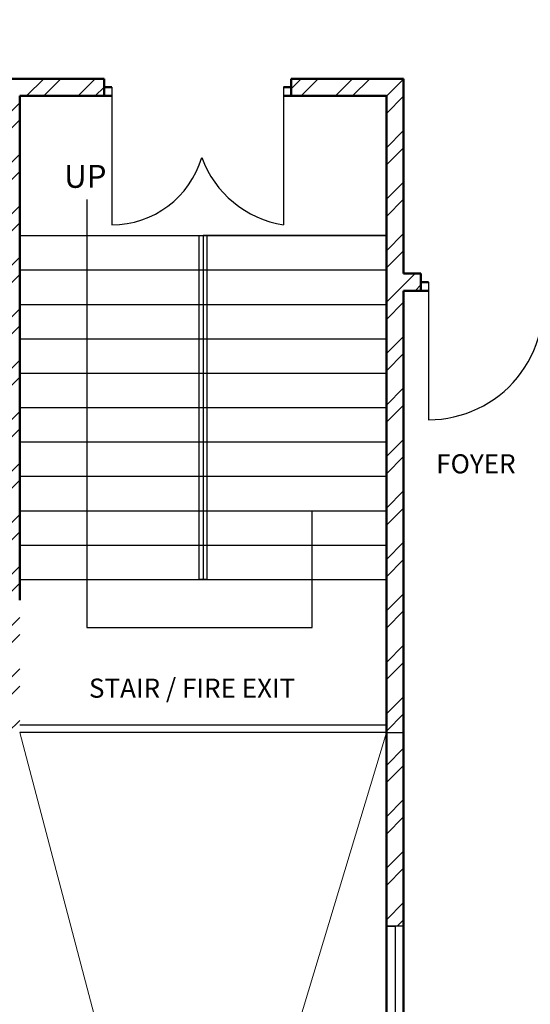
# Model space of a CAD drawing. Units: inches. Extents: x 1901 to 2863, y 888 to 2433.
# Tile 35 of 91: x 2343 to 2477, y 1474 to 1732. Entities that reach past the tile are written whole.
import ezdxf

# ---------------------------------------------------------------- set-up
doc = ezdxf.new("R2010")
doc.units = ezdxf.units.IN
for name, color, linetype, lineweight in [('A-ANNO-SYMB', 8, 'Continuous', 13), ('A-AREA-IDEN', 7, 'Continuous', 18), ('A-DOOR', 4, 'Continuous', 25), ('A-FLOR-STRS', 2, 'Continuous', 25), ('A-GLAZ', 3, 'Continuous', 25), ('A-WALL', 7, 'Continuous', 50), ('A-WALL-PATT', 8, 'Continuous', 13)]:
    doc.layers.add(name, color=color, linetype=linetype, lineweight=lineweight)
doc.styles.get("Standard").update_dxf_attribs({"font": 'arial.ttf'})

# ---------------------------------------------------------------- blocks, each defined once
blk = doc.blocks.new('WIN-60')
for p, q in [((0, 4.5), (0, 0)), ((60, 2.25), (60, 4.5)), ((60, 4.5), (60, 0)), ((0, 0), (0, 2.25)), ((0, 2.25), (60, 2.25))]:
    blk.add_line(p, q)

msp = doc.modelspace()

# ---------------------------------------------------------------- hatches: boundary and pattern name
at = {"layer": 'A-WALL-PATT'}
h = msp.add_hatch(dxfattribs=at)
h.set_pattern_fill('ANSI32', color=256)
h.paths.add_polyline_path([(2192.5, 2274.13), (2141.26, 2274.13), (2141.26, 2269.63), (2192.5, 2269.63)])
h.paths.add_polyline_path([(2259.93, 2274.13), (2216.5, 2274.13), (2216.5, 2269.63), (2255.43, 2269.63), (2255.43, 2214.63), (2250.81, 2214.63), (2250.81, 2210.13), (2259.93, 2210.13), (2259.93, 2215.13), (2271.76, 2215.13), (2271.76, 2217.38), (2271.76, 2219.63), (2259.93, 2219.63)])
h.paths.add_polyline_path([(2171.43, 2269.63), (2166.93, 2269.63), (2166.93, 2219.63), (2121.24, 2219.63), (2121.24, 2215.13), (2166.93, 2215.13), (2166.93, 2083.13), (2161.81, 2083.13), (2161.81, 2078.63), (2171.43, 2078.63), (2177, 2078.63), (2177, 2080.88), (2177, 2083.13), (2171.43, 2083.13), (2171.43, 2210.13), (2230.91, 2210.13), (2230.91, 2212.38), (2230.91, 2214.63), (2171.43, 2214.63)])
h.paths.add_polyline_path([(2117.26, 2274.13), (2089.43, 2274.13), (2089.43, 2219.63), (2081.14, 2219.63), (2081.14, 2215.13), (2089.43, 2215.13), (2098, 2215.13), (2098, 2217.38), (2098, 2219.63), (2093.93, 2219.63), (2093.93, 2269.63), (2117.26, 2269.63), (2117.26, 2271.88)])
h.paths.add_polyline_path([(2343.43, 2219.63), (2329.29, 2219.63), (2329.29, 2215.13), (2338.93, 2215.13), (2338.93, 2184.74), (2343.43, 2184.74)])
h.paths.add_polyline_path([(2338.93, 2083.13), (2329.29, 2083.13), (2208.97, 2083.13), (2208.97, 2078.63), (2338.93, 2078.63)])
h.paths.add_polyline_path([(2343.43, 2136.74), (2338.93, 2136.74), (2338.93, 1872.63), (2343.43, 1872.63)])
h.paths.add_polyline_path([(2343.43, 1863.63), (2397.68, 1863.63), (2397.68, 1821.63), (2384.14, 1821.63), (2384.14, 1812.63), (2418.33, 1812.63), (2418.33, 1817.13), (2418.33, 1821.63), (2406.68, 1821.63), (2406.68, 1863.63), (2459.5, 1863.63), (2459.5, 1821.63), (2447.14, 1821.63), (2447.14, 1812.63), (2459.5, 1812.63), (2468.5, 1812.63), (2468.5, 1872.63), (2394.43, 1872.63), (2334.43, 1872.63), (2334.43, 1812.63), (2343.43, 1812.63), (2353.25, 1812.63), (2353.25, 1821.63), (2343.43, 1821.63)])
h.paths.add_polyline_path([(2510.01, 1872.63), (2468.5, 1872.63), (2468.5, 1868.13), (2510.01, 1868.13)])
h.paths.add_polyline_path([(2514.01, 1817.13), (2468.5, 1817.13), (2468.5, 1812.63), (2482.11, 1812.63), (2482.11, 1800.61), (2486.61, 1800.61), (2486.61, 1812.63), (2514.01, 1812.63)])
h.paths.add_polyline_path([(2299.25, 1814.88), (2299.25, 1817.13), (2295.93, 1817.13), (2295.93, 1854.17), (2293.68, 1854.17), (2291.43, 1854.17), (2291.43, 1817.13), (2266.11, 1817.13), (2266.11, 1812.63), (2299.25, 1812.63)])
h.paths.add_polyline_path([(2218.11, 1817.13), (2206.46, 1817.13), (2171.43, 1817.13), (2171.43, 1949.13), (2190.1, 1949.13), (2190.1, 1953.63), (2163.47, 1953.63), (2163.47, 1949.13), (2166.93, 1949.13), (2166.93, 1817.13), (2114.3, 1817.13), (2114.3, 1812.63), (2218.11, 1812.63)])
h.paths.add_polyline_path([(2029.43, 1970.92), (2024.93, 1970.92), (2024.93, 1912.72), (2029.43, 1912.72)])
h.paths.add_polyline_path([(2132.3, 1953.63), (2113.93, 1953.63), (2113.93, 1975.89), (2111.68, 1975.89), (2109.43, 1975.89), (2109.43, 1953.63), (2029.43, 1953.63), (2029.43, 1949.13), (2132.3, 1949.13)])
h.paths.add_polyline_path([(2029.43, 1853.61), (2029.31, 1853.61), (2029.31, 1853.61), (2029.43, 1853.61), (2029.43, 1864.72), (2024.93, 1864.72), (2024.93, 1812.63), (2066.3, 1812.63), (2066.3, 1814.88), (2066.3, 1817.13), (2029.43, 1817.13)])
h.paths.add_polyline_path([(2122.93, 2010.09), (2120.68, 2010.09), (2118.43, 2010.09), (2118.43, 2006.13), (2029.43, 2006.13), (2029.43, 2001.63), (2109.43, 2001.63), (2109.43, 1998.04), (2113.93, 1998.04), (2113.93, 2001.63), (2122.93, 2001.63)])
h.paths.add_polyline_path([(2029.43, 2031.38), (2024.93, 2031.38), (2024.93, 1994.92), (2027.18, 1994.92), (2029.43, 1994.92)])
h.paths.add_polyline_path([(2029.43, 2136.74), (2024.93, 2136.74), (2024.93, 2067.38), (2027.18, 2067.38), (2029.43, 2067.38)])
h.paths.add_polyline_path([(2125.62, 2083.13), (2029.43, 2083.13), (2029.43, 2078.63), (2118.43, 2078.63), (2118.43, 2030.71), (2122.93, 2030.71), (2122.93, 2078.63), (2125.62, 2078.63)])
h.paths.add_polyline_path([(2029.43, 2215.13), (2040.47, 2215.13), (2040.47, 2217.38), (2040.47, 2219.63), (2024.93, 2219.63), (2024.93, 2184.74), (2029.43, 2184.74), (2029.43, 2187.78)])
h.paths.add_polyline_path([(2686.43, 2274.13), (2659.28, 2274.13), (2659.28, 2269.63), (2681.93, 2269.63), (2681.93, 2219.63), (2676.82, 2219.63), (2676.82, 2215.13), (2681.93, 2215.13), (2697.01, 2215.13), (2697.01, 2217.38), (2697.01, 2219.63), (2686.43, 2219.63)])
h.paths.add_polyline_path([(2609.93, 2269.63), (2635.28, 2269.63), (2635.28, 2274.13), (2571.43, 2274.13), (2571.43, 2269.63), (2605.43, 2269.63), (2605.43, 2214.63), (2549.1, 2214.63), (2549.1, 2210.13), (2605.43, 2210.13), (2605.43, 2083.13), (2601.01, 2083.13), (2601.01, 2080.88), (2601.01, 2078.63), (2609.93, 2078.63), (2616.16, 2078.63), (2616.16, 2080.88), (2616.16, 2083.13), (2609.93, 2083.13), (2609.93, 2215.13), (2651.46, 2215.13), (2651.46, 2217.38), (2651.46, 2219.63), (2609.93, 2219.63)])
h.paths.add_polyline_path([(2521.43, 2269.63), (2547.43, 2269.63), (2547.43, 2271.88), (2547.43, 2274.13), (2516.93, 2274.13), (2516.93, 2219.63), (2506.41, 2219.63), (2506.41, 2215.13), (2516.93, 2215.13), (2516.93, 2210.13), (2525.4, 2210.13), (2525.4, 2212.38), (2525.4, 2214.63), (2521.43, 2214.63)])
h.paths.add_polyline_path([(2456.01, 2219.63), (2439.43, 2219.63), (2439.43, 2187.89), (2443.93, 2187.89), (2443.93, 2215.13), (2456.01, 2215.13)])
h.paths.add_polyline_path([(2752.93, 2219.63), (2739.48, 2219.63), (2739.48, 2215.13), (2748.43, 2215.13), (2748.43, 2187.89), (2752.93, 2187.89)])
h.paths.add_polyline_path([(2752.93, 2139.89), (2748.43, 2139.89), (2748.43, 2083.13), (2648.42, 2083.13), (2648.42, 2078.63), (2654.93, 2078.63), (2654.93, 2039.44), (2659.43, 2039.44), (2659.43, 2078.63), (2748.43, 2078.63), (2748.43, 2063.43), (2752.93, 2063.43)])
h.paths.add_polyline_path([(2752.93, 2010.63), (2659.43, 2010.63), (2659.43, 2015.65), (2654.93, 2015.65), (2654.93, 2010.63), (2605.43, 2010.63), (2605.43, 1920.97), (2609.93, 1920.97), (2609.93, 2006.13), (2748.43, 2006.13), (2748.43, 1982.47), (2752.93, 1982.47)])
h.paths.add_polyline_path([(2752.93, 2027.43), (2748.43, 2027.43), (2748.43, 2010.63), (2752.93, 2010.63)])
h.paths.add_polyline_path([(2748.43, 1886.13), (2609.93, 1886.13), (2609.93, 1889.72), (2605.43, 1889.72), (2605.43, 1861.26), (2609.93, 1861.26), (2609.93, 1881.63), (2748.43, 1881.63)])
h.paths.add_polyline_path([(2456.86, 2228.83), (2498.4, 2228.83), (2498.4, 2247.49), (2456.86, 2247.49)], flags=9)
h.paths.add_polyline_path([(2038.6, 2237.42), (2080.17, 2237.42), (2080.17, 2256.08), (2038.6, 2256.08)], flags=9)
h.paths.add_polyline_path([(2292.01, 1062.39), (2539.93, 1062.39), (2539.93, 1099.49), (2292.01, 1099.49)], flags=9)
h.paths.add_polyline_path([(2424.91, 1832.25), (2448.51, 1832.25), (2448.51, 1846.68), (2424.91, 1846.68)], flags=25)
h.paths.add_polyline_path([(2359.08, 1832.25), (2382.68, 1832.25), (2382.68, 1846.68), (2359.08, 1846.68)], flags=25)
h.paths.add_polyline_path([(2352.9, 1684.8), (2367.54, 1684.8), (2367.54, 1697.17), (2352.9, 1697.17)], flags=9)
h.paths.add_polyline_path([(2079.29, 1755.83), (2169.02, 1755.83), (2169.02, 1774.37), (2079.29, 1774.37)], flags=9)
h.paths.add_polyline_path([(2404.09, 1373.86), (2404.09, 1463.59), (2385.54, 1463.59), (2385.54, 1373.86)], flags=9)
h.paths.add_polyline_path([(2268.09, 2236.37), (2309.64, 2236.37), (2309.64, 2255.03), (2268.09, 2255.03)], flags=9)
h.paths.add_polyline_path([(2575.96, 1700.95), (2665.7, 1700.95), (2665.7, 1719.5), (2575.96, 1719.5)], flags=9)
h.paths.add_polyline_path([(2302.96, 1878.47), (2329.52, 1878.47), (2329.52, 1888.78), (2302.96, 1888.78)], flags=9)
h.paths.add_polyline_path([(2097.42, 2240.58), (2126.57, 2240.58), (2126.57, 2259.23), (2097.42, 2259.23)], flags=9)
h.paths.add_polyline_path([(2208.72, 2246.12), (2237.88, 2246.12), (2237.88, 2264.78), (2208.72, 2264.78)], flags=9)
h.paths.add_polyline_path([(2038.15, 1925.96), (2076.99, 1925.96), (2076.99, 1944.62), (2038.15, 1944.62)], flags=9)
h.paths.add_polyline_path([(2239.14, 1926.67), (2288.46, 1926.67), (2288.46, 1945.33), (2239.14, 1945.33)], flags=9)
h.paths.add_polyline_path([(2175.43, 2007.33), (2212.36, 2007.33), (2212.36, 2025.99), (2175.43, 2025.99)], flags=9)
h.paths.add_polyline_path([(2225.03, 2091.79), (2263.87, 2091.79), (2263.87, 2110.45), (2225.03, 2110.45)], flags=9)
h.paths.add_polyline_path([(2035.4, 2098.48), (2074.24, 2098.48), (2074.24, 2117.14), (2035.4, 2117.14)], flags=9)
h.paths.add_polyline_path([(2050.1, 2029.21), (2083.26, 2029.21), (2083.26, 2047.87), (2050.1, 2047.87)], flags=9)
h.paths.add_polyline_path([(2069.68, 1956.72), (2098.83, 1956.72), (2098.83, 1975.38), (2069.68, 1975.38)], flags=25)
h.paths.add_polyline_path([(2328.62, 1753.34), (2361.66, 1753.34), (2361.66, 1771.99), (2328.62, 1771.99)], flags=9)
h.paths.add_polyline_path([(2395.16, 2060.89), (2395.16, 2140.65), (2378.68, 2140.65), (2378.68, 2060.89)], flags=9)
h.paths.add_polyline_path([(2463.73, 2059.02), (2492.89, 2059.02), (2492.89, 2077.68), (2463.73, 2077.68)], flags=9)
h.paths.add_polyline_path([(2458.03, 2181.54), (2496.87, 2181.54), (2496.87, 2200.19), (2458.03, 2200.19)], flags=9)
h.paths.add_polyline_path([(2527.58, 2243.07), (2556.73, 2243.07), (2556.73, 2261.73), (2527.58, 2261.73)], flags=9)
h.paths.add_polyline_path([(2694.46, 2232.77), (2736.03, 2232.77), (2736.03, 2251.42), (2694.46, 2251.42)], flags=9)
h.paths.add_polyline_path([(2637.82, 2249.22), (2666.98, 2249.22), (2666.98, 2267.88), (2637.82, 2267.88)], flags=9)
h.paths.add_polyline_path([(2623.69, 2183.54), (2662.53, 2183.54), (2662.53, 2202.2), (2623.69, 2202.2)], flags=9)
h.paths.add_polyline_path([(2691.97, 2021.5), (2725.12, 2021.5), (2725.12, 2040.16), (2691.97, 2040.16)], flags=9)
h.paths.add_polyline_path([(2621.04, 1975.91), (2662.34, 1975.91), (2662.34, 1994.57), (2621.04, 1994.57)], flags=25)
h.paths.add_polyline_path([(2479.03, 1927.62), (2519.84, 1927.62), (2519.84, 1946.28), (2479.03, 1946.28)], flags=9)
h.paths.add_polyline_path([(2670.94, 1849.08), (2716.01, 1849.08), (2716.01, 1867.73), (2670.94, 1867.73)], flags=9)
h.paths.add_polyline_path([(2523.61, 1782.96), (2550.17, 1782.96), (2550.17, 1793.26), (2523.61, 1793.26)], flags=9)
h.paths.add_polyline_path([(2450.84, 1207.33), (2492.39, 1207.33), (2492.39, 1225.99), (2450.84, 1225.99)], flags=9)
h.paths.add_polyline_path([(2527.75, 1203.84), (2556.91, 1203.84), (2556.91, 1222.5), (2527.75, 1222.5)], flags=9)
h.paths.add_polyline_path([(2639.11, 1207.2), (2668.27, 1207.2), (2668.27, 1225.86), (2639.11, 1225.86)], flags=9)
h.paths.add_polyline_path([(2692.59, 1218.97), (2734.17, 1218.97), (2734.17, 1237.62), (2692.59, 1237.62)], flags=9)
h.paths.add_polyline_path([(2669.27, 1366.33), (2708.11, 1366.33), (2708.11, 1384.99), (2669.27, 1384.99)], flags=9)
h.paths.add_polyline_path([(2463.31, 1358.03), (2502.15, 1358.03), (2502.15, 1376.69), (2463.31, 1376.69)], flags=9)
h.paths.add_polyline_path([(2494.72, 1449.96), (2531.65, 1449.96), (2531.65, 1468.62), (2494.72, 1468.62)], flags=9)
h.paths.add_polyline_path([(2675.57, 1422.16), (2708.72, 1422.16), (2708.72, 1440.81), (2675.57, 1440.81)], flags=9)
h.paths.add_polyline_path([(2685.63, 1493.89), (2714.79, 1493.89), (2714.79, 1512.55), (2685.63, 1512.55)], flags=9)
h.paths.add_polyline_path([(2686.8, 1529.91), (2725.65, 1529.91), (2725.65, 1548.57), (2686.8, 1548.57)], flags=9)
h.paths.add_polyline_path([(2503.65, 1537.99), (2552.97, 1537.99), (2552.97, 1556.65), (2503.65, 1556.65)], flags=9)
h.paths.add_polyline_path([(2291.71, 1643.5), (2318.28, 1643.5), (2318.28, 1653.81), (2291.71, 1653.81)], flags=9)
h.paths.add_polyline_path([(2450.63, 1610.52), (2477.19, 1610.52), (2477.19, 1620.82), (2450.63, 1620.82)], flags=9)
h.paths.add_polyline_path([(2359.99, 1551.81), (2422.25, 1551.81), (2422.25, 1562.12), (2359.99, 1562.12)], flags=9)
h.paths.add_polyline_path([(2280.11, 1249.01), (2321.65, 1249.01), (2321.65, 1267.66), (2280.11, 1267.66)], flags=9)
h.paths.add_polyline_path([(2164.06, 1274.23), (2193.22, 1274.23), (2193.22, 1292.89), (2164.06, 1292.89)], flags=9)
h.paths.add_polyline_path([(2118.21, 1277.69), (2151.25, 1277.69), (2151.25, 1296.35), (2118.21, 1296.35)], flags=9)
h.paths.add_polyline_path([(2031.95, 1268.53), (2073.52, 1268.53), (2073.52, 1287.19), (2031.95, 1287.19)], flags=9)
h.paths.add_polyline_path([(2050.2, 1409.08), (2089.04, 1409.08), (2089.04, 1427.74), (2050.2, 1427.74)], flags=9)
h.paths.add_polyline_path([(2243.74, 1421.03), (2282.58, 1421.03), (2282.58, 1439.69), (2243.74, 1439.69)], flags=9)
h.paths.add_polyline_path([(2190.75, 1509.77), (2231.56, 1509.77), (2231.56, 1528.43), (2190.75, 1528.43)], flags=9)
h.paths.add_polyline_path([(2058.39, 1475.42), (2091.55, 1475.42), (2091.55, 1494.07), (2058.39, 1494.07)], flags=9)
h.paths.add_polyline_path([(2062.45, 1553.09), (2091.6, 1553.09), (2091.6, 1571.75), (2062.45, 1571.75)], flags=9)
h.paths.add_polyline_path([(2219.52, 1590.37), (2266.15, 1590.37), (2266.15, 1609.02), (2219.52, 1609.02)], flags=9)
h.paths.add_polyline_path([(2041.07, 1584.19), (2079.91, 1584.19), (2079.91, 1602.85), (2041.07, 1602.85)], flags=9)
h = msp.add_hatch(dxfattribs=at)
h.set_pattern_fill('ANSI32', color=256)
h.paths.add_polyline_path([(2443.93, 2139.89), (2439.43, 2139.89), (2439.43, 2069.35), (2441.68, 2069.35), (2443.93, 2069.35), (2443.93, 2078.63), (2521.93, 2078.63), (2521.93, 2075.07), (2524.18, 2075.07), (2526.43, 2075.07), (2526.43, 2078.63), (2571.75, 2078.63), (2571.75, 2080.88), (2571.75, 2083.13), (2443.93, 2083.13)])
h.paths.add_polyline_path([(2526.43, 2054.63), (2524.18, 2054.63), (2521.93, 2054.63), (2521.93, 2030.63), (2443.93, 2030.63), (2443.93, 2045.35), (2439.43, 2045.35), (2439.43, 1983.87), (2443.93, 1983.87), (2443.93, 2026.13), (2521.93, 2026.13), (2526.43, 2026.13)])
h.paths.add_polyline_path([(2443.93, 1923.87), (2439.43, 1923.87), (2439.43, 1872.63), (2443.93, 1872.63)])
h.paths.add_polyline_path([(2636.23, 1766.13), (2609.93, 1766.13), (2609.93, 1779.79), (2605.43, 1779.79), (2605.43, 1766.13), (2486.61, 1766.13), (2486.61, 1770.67), (2482.11, 1770.67), (2482.11, 1766.13), (2482.11, 1761.63), (2636.23, 1761.63), (2636.23, 1763.88)])
h.paths.add_polyline_path([(2519.54, 1663.38), (2519.54, 1665.63), (2494.93, 1665.63), (2481.83, 1665.63), (2481.83, 1663.38), (2481.83, 1661.13), (2490.43, 1661.13), (2490.43, 1640.16), (2494.93, 1640.16), (2494.93, 1661.13), (2519.54, 1661.13)])
h.paths.add_polyline_path([(2443.93, 1712.13), (2443.93, 1716.63), (2414.46, 1716.63), (2414.46, 1712.13), (2439.43, 1712.13), (2439.43, 1545.51), (2443.93, 1545.51), (2443.93, 1661.13), (2448.47, 1661.13), (2448.47, 1665.63), (2443.93, 1665.63)])
h.paths.add_polyline_path([(2343.43, 1712.13), (2365.52, 1712.13), (2365.52, 1714.38), (2365.52, 1716.63), (2333.87, 1716.63), (2333.87, 1714.38), (2333.87, 1712.13), (2338.93, 1712.13), (2338.93, 1575.63), (2338.93, 1545.51), (2343.43, 1545.51), (2343.43, 1547.51), (2343.43, 1580.13)])
h.paths.add_polyline_path([(2752.93, 1665.63), (2579.54, 1665.63), (2579.54, 1661.13), (2615.93, 1661.13), (2615.93, 1529.13), (2598.93, 1529.13), (2598.93, 1524.63), (2623.13, 1524.63), (2623.13, 1526.88), (2623.13, 1529.13), (2620.43, 1529.13), (2620.43, 1661.13), (2748.43, 1661.13), (2748.43, 1633.5), (2752.93, 1633.5)])
h.paths.add_polyline_path([(2752.93, 1419.93), (2748.43, 1419.93), (2748.43, 1400.13), (2659.43, 1400.13), (2659.43, 1444.33), (2657.18, 1444.33), (2654.93, 1444.33), (2654.93, 1400.13), (2643.65, 1400.13), (2643.65, 1395.63), (2748.43, 1395.63), (2748.43, 1364.04), (2752.93, 1364.04)])
h.paths.add_polyline_path([(2752.93, 1492.88), (2748.43, 1492.88), (2748.43, 1476.63), (2667.43, 1476.63), (2667.43, 1479.71), (2665.18, 1479.71), (2662.93, 1479.71), (2662.93, 1476.63), (2654.93, 1476.63), (2654.93, 1469.54), (2659.43, 1469.54), (2659.43, 1472.13), (2748.43, 1472.13), (2748.43, 1455.93), (2752.93, 1455.93)])
h.paths.add_polyline_path([(2752.93, 1304.04), (2748.43, 1304.04), (2748.43, 1263.63), (2738.66, 1263.63), (2738.66, 1259.13), (2752.93, 1259.13)])
h.paths.add_polyline_path([(2685.93, 1259.13), (2695.49, 1259.13), (2695.49, 1261.38), (2695.49, 1263.63), (2677.84, 1263.63), (2677.84, 1261.38), (2677.84, 1259.13), (2681.43, 1259.13), (2681.43, 1203.63), (2653.28, 1203.63), (2653.28, 1199.13), (2685.93, 1199.13), (2685.93, 1203.63)])
h.paths.add_polyline_path([(2609.43, 1395.63), (2611.85, 1395.63), (2611.85, 1400.13), (2598.89, 1400.13), (2598.89, 1397.88), (2598.89, 1395.63), (2604.93, 1395.63), (2604.93, 1268.13), (2554.73, 1268.13), (2554.73, 1265.88), (2554.73, 1263.63), (2604.93, 1263.63), (2604.93, 1203.63), (2571.31, 1203.63), (2571.31, 1199.13), (2604.93, 1199.13), (2629.28, 1199.13), (2629.28, 1201.38), (2629.28, 1203.63), (2609.43, 1203.63), (2609.43, 1258.63), (2609.43, 1259.13), (2654.8, 1259.13), (2654.8, 1263.63), (2609.43, 1263.63)])
h.paths.add_polyline_path([(2443.93, 1304.04), (2439.43, 1304.04), (2439.43, 1259.13), (2443.93, 1259.13), (2456.16, 1259.13), (2456.16, 1261.38), (2456.16, 1263.63), (2443.93, 1263.63)])
h.paths.add_polyline_path([(2525.43, 1263.63), (2531.78, 1263.63), (2531.78, 1268.13), (2520.93, 1268.13), (2520.93, 1263.63), (2511.41, 1263.63), (2511.41, 1259.13), (2520.93, 1259.13), (2520.93, 1199.13), (2547.31, 1199.13), (2547.31, 1201.38), (2547.31, 1203.63), (2525.43, 1203.63)])
h.paths.add_polyline_path([(2443.93, 1434.84), (2439.43, 1434.84), (2439.43, 1364.04), (2441.68, 1364.04), (2443.93, 1364.04)])
h.paths.add_polyline_path([(2567.13, 1400.13), (2443.93, 1400.13), (2443.93, 1395.63), (2567.13, 1395.63)])
h.paths.add_polyline_path([(2443.93, 1545.51), (2439.43, 1545.51), (2439.43, 1494.84), (2443.93, 1494.84)])
h.paths.add_polyline_path([(2494.93, 1553.35), (2492.68, 1553.35), (2490.43, 1553.35), (2490.43, 1524.63), (2494.93, 1524.63), (2525.94, 1524.63), (2525.94, 1526.88), (2525.94, 1529.13), (2494.93, 1529.13)])
h.paths.add_polyline_path([(2752.93, 1573.5), (2748.43, 1573.5), (2748.43, 1529.13), (2657.76, 1529.13), (2657.76, 1524.63), (2662.93, 1524.63), (2662.93, 1498.63), (2667.43, 1498.63), (2667.43, 1524.63), (2748.43, 1524.63), (2748.43, 1516.88), (2752.93, 1516.88)])
h.paths.add_polyline_path([(2038.6, 2237.42), (2080.17, 2237.42), (2080.17, 2256.08), (2038.6, 2256.08)], flags=9)
h.paths.add_polyline_path([(2292.01, 1062.39), (2539.93, 1062.39), (2539.93, 1099.49), (2292.01, 1099.49)], flags=9)
h.paths.add_polyline_path([(2424.91, 1832.25), (2448.51, 1832.25), (2448.51, 1846.68), (2424.91, 1846.68)], flags=9)
h.paths.add_polyline_path([(2359.08, 1832.25), (2382.68, 1832.25), (2382.68, 1846.68), (2359.08, 1846.68)], flags=9)
h.paths.add_polyline_path([(2352.9, 1684.8), (2367.54, 1684.8), (2367.54, 1697.17), (2352.9, 1697.17)], flags=9)
h.paths.add_polyline_path([(2079.29, 1755.83), (2169.02, 1755.83), (2169.02, 1774.37), (2079.29, 1774.37)], flags=9)
h.paths.add_polyline_path([(2404.09, 1373.86), (2404.09, 1463.59), (2385.54, 1463.59), (2385.54, 1373.86)], flags=9)
h.paths.add_polyline_path([(2268.09, 2236.37), (2309.64, 2236.37), (2309.64, 2255.03), (2268.09, 2255.03)], flags=9)
h.paths.add_polyline_path([(2575.96, 1700.95), (2665.7, 1700.95), (2665.7, 1719.5), (2575.96, 1719.5)], flags=9)
h.paths.add_polyline_path([(2302.96, 1878.47), (2329.52, 1878.47), (2329.52, 1888.78), (2302.96, 1888.78)], flags=9)
h.paths.add_polyline_path([(2097.42, 2240.58), (2126.57, 2240.58), (2126.57, 2259.23), (2097.42, 2259.23)], flags=9)
h.paths.add_polyline_path([(2208.72, 2246.12), (2237.88, 2246.12), (2237.88, 2264.78), (2208.72, 2264.78)], flags=9)
h.paths.add_polyline_path([(2038.15, 1925.96), (2076.99, 1925.96), (2076.99, 1944.62), (2038.15, 1944.62)], flags=9)
h.paths.add_polyline_path([(2239.14, 1926.67), (2288.46, 1926.67), (2288.46, 1945.33), (2239.14, 1945.33)], flags=9)
h.paths.add_polyline_path([(2175.43, 2007.33), (2212.36, 2007.33), (2212.36, 2025.99), (2175.43, 2025.99)], flags=9)
h.paths.add_polyline_path([(2225.03, 2091.79), (2263.87, 2091.79), (2263.87, 2110.45), (2225.03, 2110.45)], flags=9)
h.paths.add_polyline_path([(2035.4, 2098.48), (2074.24, 2098.48), (2074.24, 2117.14), (2035.4, 2117.14)], flags=9)
h.paths.add_polyline_path([(2050.1, 2029.21), (2083.26, 2029.21), (2083.26, 2047.87), (2050.1, 2047.87)], flags=9)
h.paths.add_polyline_path([(2069.68, 1956.72), (2098.83, 1956.72), (2098.83, 1975.38), (2069.68, 1975.38)], flags=9)
h.paths.add_polyline_path([(2328.62, 1753.34), (2361.66, 1753.34), (2361.66, 1771.99), (2328.62, 1771.99)], flags=9)
h.paths.add_polyline_path([(2395.16, 2060.89), (2395.16, 2140.65), (2378.68, 2140.65), (2378.68, 2060.89)], flags=9)
h.paths.add_polyline_path([(2463.73, 2059.02), (2492.89, 2059.02), (2492.89, 2077.68), (2463.73, 2077.68)], flags=9)
h.paths.add_polyline_path([(2458.03, 2181.54), (2496.87, 2181.54), (2496.87, 2200.19), (2458.03, 2200.19)], flags=9)
h.paths.add_polyline_path([(2456.86, 2228.83), (2498.4, 2228.83), (2498.4, 2247.49), (2456.86, 2247.49)], flags=9)
h.paths.add_polyline_path([(2527.58, 2243.07), (2556.73, 2243.07), (2556.73, 2261.73), (2527.58, 2261.73)], flags=9)
h.paths.add_polyline_path([(2694.46, 2232.77), (2736.03, 2232.77), (2736.03, 2251.42), (2694.46, 2251.42)], flags=9)
h.paths.add_polyline_path([(2637.82, 2249.22), (2666.98, 2249.22), (2666.98, 2267.88), (2637.82, 2267.88)], flags=9)
h.paths.add_polyline_path([(2623.69, 2183.54), (2662.53, 2183.54), (2662.53, 2202.2), (2623.69, 2202.2)], flags=9)
h.paths.add_polyline_path([(2691.97, 2021.5), (2725.12, 2021.5), (2725.12, 2040.16), (2691.97, 2040.16)], flags=9)
h.paths.add_polyline_path([(2621.04, 1975.91), (2662.34, 1975.91), (2662.34, 1994.57), (2621.04, 1994.57)], flags=9)
h.paths.add_polyline_path([(2479.03, 1927.62), (2519.84, 1927.62), (2519.84, 1946.28), (2479.03, 1946.28)], flags=9)
h.paths.add_polyline_path([(2670.94, 1849.08), (2716.01, 1849.08), (2716.01, 1867.73), (2670.94, 1867.73)], flags=9)
h.paths.add_polyline_path([(2523.61, 1782.96), (2550.17, 1782.96), (2550.17, 1793.26), (2523.61, 1793.26)], flags=9)
h.paths.add_polyline_path([(2450.84, 1207.33), (2492.39, 1207.33), (2492.39, 1225.99), (2450.84, 1225.99)], flags=9)
h.paths.add_polyline_path([(2527.75, 1203.84), (2556.91, 1203.84), (2556.91, 1222.5), (2527.75, 1222.5)], flags=9)
h.paths.add_polyline_path([(2639.11, 1207.2), (2668.27, 1207.2), (2668.27, 1225.86), (2639.11, 1225.86)], flags=9)
h.paths.add_polyline_path([(2692.59, 1218.97), (2734.17, 1218.97), (2734.17, 1237.62), (2692.59, 1237.62)], flags=9)
h.paths.add_polyline_path([(2669.27, 1366.33), (2708.11, 1366.33), (2708.11, 1384.99), (2669.27, 1384.99)], flags=25)
h.paths.add_polyline_path([(2463.31, 1358.03), (2502.15, 1358.03), (2502.15, 1376.69), (2463.31, 1376.69)], flags=9)
h.paths.add_polyline_path([(2494.72, 1449.96), (2531.65, 1449.96), (2531.65, 1468.62), (2494.72, 1468.62)], flags=9)
h.paths.add_polyline_path([(2675.57, 1422.16), (2708.72, 1422.16), (2708.72, 1440.81), (2675.57, 1440.81)], flags=25)
h.paths.add_polyline_path([(2685.63, 1493.89), (2714.79, 1493.89), (2714.79, 1512.55), (2685.63, 1512.55)], flags=9)
h.paths.add_polyline_path([(2686.8, 1529.91), (2725.65, 1529.91), (2725.65, 1548.57), (2686.8, 1548.57)], flags=25)
h.paths.add_polyline_path([(2503.65, 1537.99), (2552.97, 1537.99), (2552.97, 1556.65), (2503.65, 1556.65)], flags=9)
h.paths.add_polyline_path([(2291.71, 1643.5), (2318.28, 1643.5), (2318.28, 1653.81), (2291.71, 1653.81)], flags=9)
h.paths.add_polyline_path([(2450.63, 1610.52), (2477.19, 1610.52), (2477.19, 1620.82), (2450.63, 1620.82)], flags=9)
h.paths.add_polyline_path([(2359.99, 1551.81), (2422.25, 1551.81), (2422.25, 1562.12), (2359.99, 1562.12)], flags=9)
h.paths.add_polyline_path([(2280.11, 1249.01), (2321.65, 1249.01), (2321.65, 1267.66), (2280.11, 1267.66)], flags=9)
h.paths.add_polyline_path([(2164.06, 1274.23), (2193.22, 1274.23), (2193.22, 1292.89), (2164.06, 1292.89)], flags=9)
h.paths.add_polyline_path([(2118.21, 1277.69), (2151.25, 1277.69), (2151.25, 1296.35), (2118.21, 1296.35)], flags=9)
h.paths.add_polyline_path([(2031.95, 1268.53), (2073.52, 1268.53), (2073.52, 1287.19), (2031.95, 1287.19)], flags=9)
h.paths.add_polyline_path([(2050.2, 1409.08), (2089.04, 1409.08), (2089.04, 1427.74), (2050.2, 1427.74)], flags=9)
h.paths.add_polyline_path([(2243.74, 1421.03), (2282.58, 1421.03), (2282.58, 1439.69), (2243.74, 1439.69)], flags=9)
h.paths.add_polyline_path([(2190.75, 1509.77), (2231.56, 1509.77), (2231.56, 1528.43), (2190.75, 1528.43)], flags=9)
h.paths.add_polyline_path([(2058.39, 1475.42), (2091.55, 1475.42), (2091.55, 1494.07), (2058.39, 1494.07)], flags=9)
h.paths.add_polyline_path([(2062.45, 1553.09), (2091.6, 1553.09), (2091.6, 1571.75), (2062.45, 1571.75)], flags=9)
h.paths.add_polyline_path([(2219.52, 1590.37), (2266.15, 1590.37), (2266.15, 1609.02), (2219.52, 1609.02)], flags=9)
h.paths.add_polyline_path([(2041.07, 1584.19), (2079.91, 1584.19), (2079.91, 1602.85), (2041.07, 1602.85)], flags=9)

# ---------------------------------------------------------------- linework, layer by layer
at = {"layer": 'A-ANNO-SYMB'}
for p, q in [((2343.43, 1228.13), (2439.43, 1545.51)), ((2343.43, 1545.51), (2439.43, 1181.13))]:
    msp.add_line(p, q, dxfattribs=at)
at = {"layer": 'A-DOOR'}
for p, q in [((2367.52, 1714.38), (2367.52, 1678.38)), ((2412.46, 1714.38), (2412.46, 1678.38)), ((2450.47, 1663.38), (2450.47, 1627.38))]:
    msp.add_line(p, q, dxfattribs=at)
for centre, radius, start, end in [((2367.52, 1702.92), 24.53, 270, 343.6931), ((2416.77, 1705.39), 27.35, 200.0258, 260.9451), ((2450.47, 1657.35), 29.97, 270, 11.6082)]:
    msp.add_arc(centre, radius, start, end, dxfattribs=at)
at = {"layer": 'A-FLOR-STRS'}
for p, q in [((2360.98, 1685.01), (2360.98, 1573.01)), ((2343.43, 1675.58), (2439.43, 1675.58)), ((2390.43, 1585.58), (2390.43, 1675.58)), ((2390.43, 1675.58), (2391.43, 1675.58)), ((2439.43, 1675.58), (2391.43, 1675.58)), ((2391.43, 1675.58), (2391.43, 1585.58)), ((2391.43, 1675.58), (2392.43, 1675.58)), ((2392.43, 1675.58), (2392.43, 1585.58)), ((2343.43, 1666.58), (2439.43, 1666.58)), ((2343.43, 1657.58), (2439.43, 1657.58)), ((2343.43, 1648.58), (2439.43, 1648.58)), ((2343.43, 1639.58), (2439.43, 1639.58)), ((2343.43, 1630.58), (2439.43, 1630.58)), ((2343.43, 1621.58), (2439.43, 1621.58)), ((2343.43, 1612.58), (2439.43, 1612.58)), ((2343.43, 1603.58), (2439.43, 1603.58)), ((2420.01, 1573.01), (2420.01, 1603.58)), ((2343.43, 1594.58), (2439.43, 1594.58)), ((2343.43, 1585.58), (2439.43, 1585.58)), ((2391.43, 1585.58), (2390.43, 1585.58)), ((2392.43, 1585.58), (2391.43, 1585.58)), ((2360.98, 1573.01), (2420.01, 1573.01)), ((2343.43, 1547.51), (2439.43, 1547.51)), ((2439.43, 1545.51), (2343.43, 1545.51)), ((2439.43, 1545.51), (2443.93, 1545.51))]:
    msp.add_line(p, q, dxfattribs=at)
at = {"layer": 'A-WALL'}
for p, q in [((2333.87, 1716.63), (2365.52, 1716.63)), ((2365.52, 1716.63), (2365.52, 1712.13)), ((2414.46, 1716.63), (2414.46, 1712.13)), ((2414.46, 1716.63), (2443.93, 1716.63)), ((2443.93, 1716.63), (2443.93, 1712.13)), ((2365.52, 1712.13), (2365.52, 1714.38)), ((2365.52, 1714.38), (2367.52, 1714.38)), ((2414.46, 1714.38), (2412.46, 1714.38)), ((2414.46, 1712.13), (2414.46, 1714.38)), ((2343.43, 1712.13), (2343.43, 1580.13)), ((2367.52, 1712.13), (2343.43, 1712.13)), ((2439.43, 1712.13), (2412.46, 1712.13)), ((2439.43, 1259.13), (2439.43, 1712.13)), ((2443.93, 1712.13), (2443.93, 1665.63)), ((2448.47, 1665.63), (2443.93, 1665.63)), ((2448.47, 1661.13), (2448.47, 1665.63)), ((2448.47, 1665.63), (2448.47, 1663.38)), ((2448.47, 1663.38), (2450.47, 1663.38)), ((2443.93, 1661.13), (2450.47, 1661.13)), ((2443.93, 1661.13), (2443.93, 1263.63))]:
    msp.add_line(p, q, dxfattribs=at)

# ---------------------------------------------------------------- block references
at = {"layer": 'A-GLAZ', "rotation": 270.0000000000005}
msp.add_blockref('WIN-60', (2439.43, 1494.84), dxfattribs=at)

# ---------------------------------------------------------------- texts
at = {"layer": 'A-AREA-IDEN', "char_height": 5, "attachment_point": 1}
for s, width, insert in [('FOYER', 105.9592, (2452.45, 1618.34)), ('STAIR / FIRE EXIT', 95.4451, (2361.55, 1559.63))]:
    msp.add_mtext_dynamic_manual_height_columns(s, width=width, gutter_width=12.5, heights=[0], dxfattribs=dict(at, insert=insert))
at = {"layer": 'A-FLOR-STRS', "insert": (2355.06, 1694.08), "char_height": 6, "attachment_point": 1}
msp.add_mtext_dynamic_manual_height_columns('UP', width=33.7572, gutter_width=12.5, heights=[2.6], dxfattribs=at)

doc.saveas('drawing.dxf')
